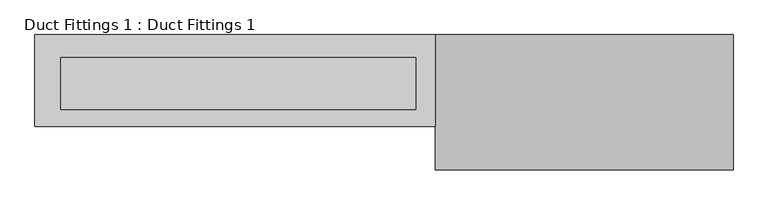
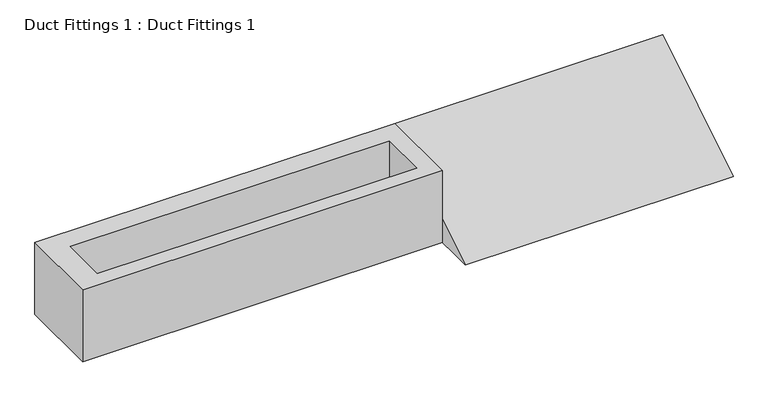
"""IFC4 building model written with IfcOpenShell, lengths in millimetres: duct fitting geometry, Duct Fittings 1 : Duct Fittings 1."""

from ifc_helpers import new_model, si_unit, frame, origin, place, context, project, spatial, polyline, outline, extrude, faceted_brep, source, transform, mapped, element, save


def duct_fittings_1_duct_fittings_1_d2289eb8(model_context):
    return source(origin(), model_context, "Body", "SolidModel", [
        faceted_brep([(-11637.4667042, -6210.1296146, 1876.3331333), (-6315.8667042, -6210.1296146, 1876.3331333), (-6315.8667042, -6210.1296146, 3000.0), (-11637.4667042, -6210.1296146, 3000.0), (-11637.4667042, -4990.9296146, 1876.3331333), (-11637.4667042, -4990.9296146, 3000.0), (-6315.8667042, -4990.9296146, 3000.0), (-6315.8667042, -4990.9296146, 1876.3331333), (-6571.4314791, -5295.7296146, 3000.0), (-6571.4314791, -5987.9368948, 3000.0), (-11294.3425766, -5987.9368948, 3000.0), (-11294.3425766, -5295.7296146, 3000.0), (-6571.4314791, -5295.7296146, 2413.9215363), (-11294.3425766, -5295.7296146, 2413.9215363), (-11294.3425766, -5987.9368948, 2413.9215363), (-6571.4314791, -5987.9368948, 2413.9215363)], [[[0, 1, 2, 3]], [[4, 5, 6, 7]], [[1, 0, 4, 7]], [[2, 1, 7, 6]], [[3, 2, 6, 5], [8, 9, 10, 11]], [[0, 3, 5, 4]], [[12, 13, 14, 15]], [[12, 15, 9, 8]], [[15, 14, 10, 9]], [[14, 13, 11, 10]], [[13, 12, 8, 11]]]),
        extrude(outline(polyline([(-4990.9296146, 3000.0), (-4990.9296146, 1876.3331333), (-6789.1725006, 1876.3331333), (-4990.9296146, 3000.0)])), frame((-6315.8667042, 0.0, 0.0), z_axis=(1.0, 0.0, 0.0), x_axis=(0.0, 1.0, 0.0)), (0.0, 0.0, 1.0), 3962.4),
    ])


if __name__ == "__main__":
    model = new_model("IFC4")
    model_context = context("Model", 3, world=origin())
    ifc_project = project(units=[si_unit("LENGTHUNIT", "METRE", prefix="MILLI")], contexts=[model_context])
    site = spatial("IfcSite", under=ifc_project)
    building = spatial("IfcBuilding", under=site)
    placement = place(None, origin())
    duct_fittings_1_duct_fittings_1_shape = duct_fittings_1_duct_fittings_1_d2289eb8(model_context)
    element("IfcDuctFitting", 1, ObjectType="Duct Fittings 1 : Duct Fittings 1", at=placement, inside=building, context=model_context, shape_type="MappedRepresentation", body=[
        mapped(duct_fittings_1_duct_fittings_1_shape, transform((0.0, 0.0, 0.0), x_axis=(1.0, 0.0, 0.0), y_axis=(0.0, 1.0, 0.0), z_axis=(0.0, 0.0, 1.0))),
    ])
    save(model, "model.ifc")

# Revit data of these elements
# Element 1 (IfcDuctFitting, "Duct Fittings 1 : Duct Fittings 1")
#   Materials on its faces: "RC"
# Materials
#   "RC": class "Generic", colour RGB 255 255 255, transparency 0, Cost = 0
